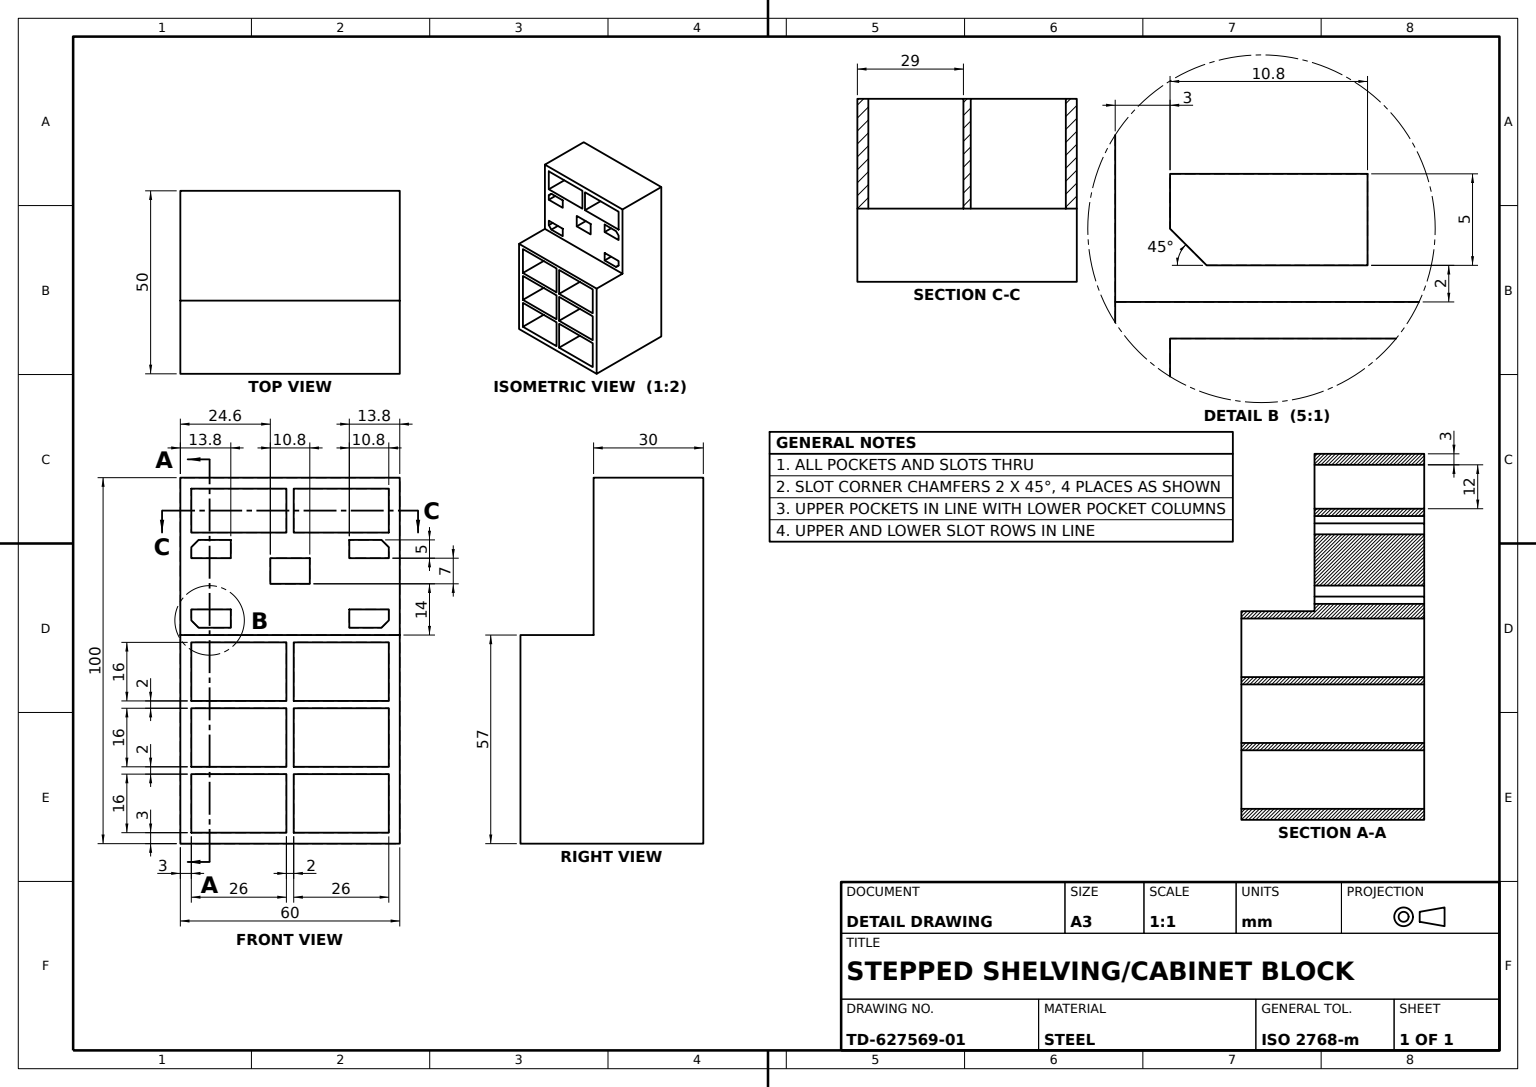
from build123d import *

# Parameters (mm, degrees)
BASE_BLOCK_SKETCH_W         = 60
BASE_BLOCK_SKETCH_H         = 100
BASE_BLOCK_DEPTH            = 30
LOWER_CELL_POCKETS_SKETCH_W = 26
LOWER_CELL_POCKETS_SKETCH_H = 12
LOWER_CELL_POCKETS_DEPTH    = 66.574385243
UPPER_STEP_SKETCH_W         = 60
UPPER_STEP_SKETCH_H         = 57
UPPER_STEP_BOSS_DEPTH       = 20
UPPER_CELL_POCKETS_SKETCH_W = 26
UPPER_CELL_POCKETS_SKETCH_H = 16
UPPER_CELL_POCKETS_DEPTH    = 77.811457479
BACK_WALL_SLOTS_SKETCH_W    = 10.8
BACK_WALL_SLOTS_SKETCH_H    = 7
BACK_WALL_SLOTS_DEPTH       = 66.574385243


with BuildPart() as part:
    # Base Block Sketch → Base Block (new body)
    with BuildSketch(Plane.XY):
        Rectangle(BASE_BLOCK_SKETCH_W, BASE_BLOCK_SKETCH_H)
    extrude(amount=BASE_BLOCK_DEPTH)

    # Lower Cell Pockets Sketch → Lower Cell Pockets (cut, through all)
    with BuildSketch(Plane.XY.offset(30)):
        with Locations((14, 41)):
            Rectangle(LOWER_CELL_POCKETS_SKETCH_W, LOWER_CELL_POCKETS_SKETCH_H)
        Polygon((-21.788065722, 47), (-27, 47), (-27, 35), (-1, 35), (-1, 47), align=None)
    extrude(amount=-LOWER_CELL_POCKETS_DEPTH, mode=Mode.SUBTRACT)

    # Upper Step Sketch → Upper Step Boss (add)
    with BuildSketch(Plane.XY.offset(30)):
        with Locations((0, -21.5)):
            Rectangle(UPPER_STEP_SKETCH_W, UPPER_STEP_SKETCH_H)
    extrude(amount=UPPER_STEP_BOSS_DEPTH)

    # Upper Cell Pockets Sketch → Upper Cell Pockets (cut, through all)
    with BuildSketch(Plane.XY.offset(50)):
        with Locations((-14, -3)):
            Rectangle(UPPER_CELL_POCKETS_SKETCH_W, UPPER_CELL_POCKETS_SKETCH_H)
        with Locations((14, -3)):
            Rectangle(UPPER_CELL_POCKETS_SKETCH_W, UPPER_CELL_POCKETS_SKETCH_H)
        with Locations((14, -21)):
            Rectangle(UPPER_CELL_POCKETS_SKETCH_W, UPPER_CELL_POCKETS_SKETCH_H)
        with Locations((14, -39)):
            Rectangle(UPPER_CELL_POCKETS_SKETCH_W, UPPER_CELL_POCKETS_SKETCH_H)
        with Locations((-14, -21)):
            Rectangle(UPPER_CELL_POCKETS_SKETCH_W, UPPER_CELL_POCKETS_SKETCH_H)
        with Locations((-14, -39)):
            Rectangle(UPPER_CELL_POCKETS_SKETCH_W, UPPER_CELL_POCKETS_SKETCH_H)
    extrude(amount=-UPPER_CELL_POCKETS_DEPTH, mode=Mode.SUBTRACT)

    # Back Wall Slots Sketch → Back Wall Slots (cut, through all)
    with BuildSketch(Plane.XY.offset(30)):
        Polygon((27, 14), (16.2, 14), (16.2, 9), (25, 9), (27, 11), align=None)
        with Locations((0, 24.5)):
            Rectangle(BACK_WALL_SLOTS_SKETCH_W, BACK_WALL_SLOTS_SKETCH_H)
        Polygon((-16.2, 33), (-25, 33), (-27, 31), (-27, 28), (-16.2, 28), align=None)
        Polygon((25, 33), (16.2, 33), (16.2, 28), (27, 28), (27, 31), align=None)
        Polygon((-16.2, 14), (-27, 14), (-27, 11), (-25, 9), (-16.2, 9), align=None)
    extrude(amount=-BACK_WALL_SLOTS_DEPTH, mode=Mode.SUBTRACT)


solid = part.part
